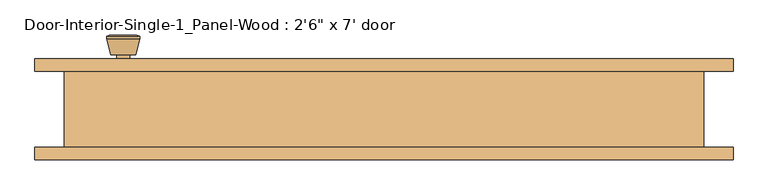
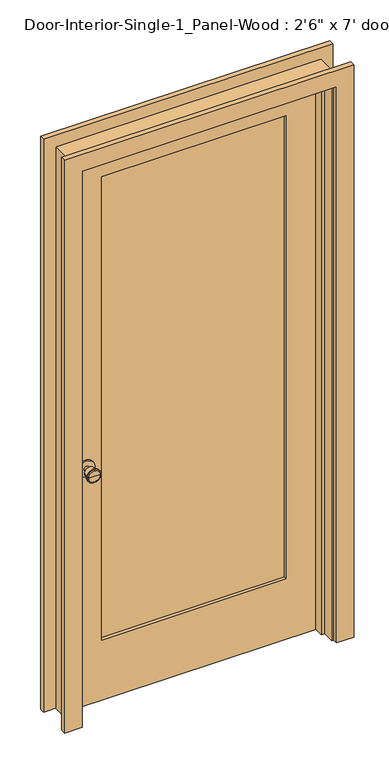
"""IFC4 building model written with IfcOpenShell, lengths in millimetres: door geometry."""

from ifc_helpers import new_model, si_unit, point, frame, frame_2d, origin, place, context, project, spatial, polyline, circle_curve, trimmed, segment, composite_curve, outline, extrude, faceted_brep, source, transform, mapped, element, save
from ifc_brep_helpers import plane_surface, cylinder_surface, revolved_surface, advanced_brep


def door_3c6ab76a(model_context):
    return source(origin(), model_context, "Body", "SolidModel", [
        advanced_brep(
        [(-393.7, 13.05, 914.4), (-383.7, 13.05, 914.4), (-403.7, 13.05, 914.4), (-373.2241324, -35.95, 914.4), (-393.7, -35.95, 914.4), (-414.1758676, -35.95, 914.4), (-368.7, -34.1221319, 914.4), (-418.7, -34.1221319, 914.4), (-368.7, -30.6584537, 914.4), (-418.7, -30.6584537, 914.4), (-375.063764, -5.95, 914.4), (-412.336236, -5.95, 914.4), (-383.7, -5.95, 914.4), (-403.7, -5.95, 914.4)],
        [
            (0, 1),
            (1, 2, circle_curve(frame((-393.7, 13.05, 914.4), z_axis=(0.0, 1.0, 0.0), x_axis=(-1.0, 0.0, 0.0)), 10.0)),
            (2, 0),
            (2, 1, circle_curve(frame((-393.7, 13.05, 914.4), z_axis=(0.0, 1.0, 0.0), x_axis=(-1.0, 0.0, 0.0)), 10.0)),
            (3, 4),
            (4, 5),
            (5, 3, circle_curve(frame((-393.7, -35.95, 914.4), z_axis=(0.0, -1.0, 0.0), x_axis=(-1.0, 0.0, 0.0)), 20.4758676)),
            (3, 5, circle_curve(frame((-393.7, -35.95, 914.4), z_axis=(0.0, -1.0, 0.0), x_axis=(-1.0, 0.0, 0.0)), 20.4758676)),
            (6, 3),
            (5, 7),
            (7, 6, circle_curve(frame((-393.7, -34.1221319, 914.4), z_axis=(0.0, -1.0, 0.0), x_axis=(-1.0, 0.0, 0.0)), 25.0)),
            (6, 7, circle_curve(frame((-393.7, -34.1221319, 914.4), z_axis=(0.0, -1.0, 0.0), x_axis=(-1.0, 0.0, 0.0)), 25.0)),
            (8, 6),
            (7, 9),
            (9, 8, circle_curve(frame((-393.7, -30.6584537, 914.4), z_axis=(0.0, -1.0, 0.0), x_axis=(-1.0, 0.0, 0.0)), 25.0)),
            (8, 9, circle_curve(frame((-393.7, -30.6584537, 914.4), z_axis=(0.0, -1.0, 0.0), x_axis=(-1.0, 0.0, 0.0)), 25.0)),
            (10, 8),
            (9, 11),
            (11, 10, circle_curve(frame((-393.7, -5.95, 914.4), z_axis=(0.0, -1.0, 0.0), x_axis=(-1.0, 0.0, 0.0)), 18.636236)),
            (10, 11, circle_curve(frame((-393.7, -5.95, 914.4), z_axis=(0.0, -1.0, 0.0), x_axis=(-1.0, 0.0, 0.0)), 18.636236)),
            (12, 10),
            (11, 13),
            (13, 12, circle_curve(frame((-393.7, -5.95, 914.4), z_axis=(0.0, -1.0, 0.0), x_axis=(-1.0, 0.0, 0.0)), 10.0)),
            (12, 13, circle_curve(frame((-393.7, -5.95, 914.4), z_axis=(0.0, -1.0, 0.0), x_axis=(-1.0, 0.0, 0.0)), 10.0)),
            (1, 12),
            (13, 2),
        ],
        [
            plane_surface(frame((-393.7, 13.05, 914.4), z_axis=(0.0, 1.0, 0.0), x_axis=(-1.0, 0.0, 0.0))),
            plane_surface(frame((-393.7, -35.95, 914.4), z_axis=(0.0, -1.0, 0.0), x_axis=(-1.0, 0.0, 0.0))),
            revolved_surface(polyline([(-414.1758676, -35.95, 914.4), (-418.7, -34.1221319, 914.4)]), (-393.7, 13.05, 914.4), (0.0, 1.0, 0.0)),
            cylinder_surface(frame((-393.7, 13.05, 914.4), z_axis=(0.0, 1.0, 0.0), x_axis=(-1.0, 0.0, 0.0)), 25.0),
            revolved_surface(polyline([(-418.7, -30.6584537, 914.4), (-412.336236, -5.95, 914.4)]), (-393.7, 13.05, 914.4), (0.0, 1.0, 0.0)),
            plane_surface(frame((-393.7, -5.95, 914.4), z_axis=(0.0, 1.0, 0.0), x_axis=(-1.0, 0.0, 0.0))),
            cylinder_surface(frame((-393.7, 13.05, 914.4), z_axis=(0.0, 1.0, 0.0), x_axis=(-1.0, 0.0, 0.0)), 10.0),
        ],
        [
            (0, [[1, 2, 3]]),
            (0, [[-3, 4, -1]]),
            (1, [[5, 6, 7]]),
            (1, [[-6, -5, 8]]),
            (2, [[9, -7, 10, 11]]),
            (2, [[-10, -8, -9, 12]]),
            (3, [[13, -11, 14, 15]]),
            (3, [[-14, -12, -13, 16]]),
            (4, [[17, -15, 18, 19]]),
            (4, [[-18, -16, -17, 20]]),
            (5, [[21, -19, 22, 23]]),
            (5, [[-22, -20, -21, 24]]),
            (6, [[25, -23, 26, -2]]),
            (6, [[-26, -24, -25, -4]]),
        ],
    ),
        extrude(outline(composite_curve([segment(trimmed(circle_curve(frame_2d((914.4, -393.7)), 30.0), [point((914.4, -423.7))], [point((914.4, -363.7))], False, "CARTESIAN"), True, "CONTINUOUS"), segment(trimmed(circle_curve(frame_2d((914.4, -393.7)), 30.0), [point((914.4, -363.7))], [point((914.4, -423.7))], False, "CARTESIAN"), True, "CONTINUOUS")], self_intersect=False)), frame((0.0, 13.05, 0.0), z_axis=(0.0, 1.0, 0.0), x_axis=(0.0, 0.0, 1.0)), (0.0, 0.0, 1.0), 6.0),
        advanced_brep(
        [(-393.7, 59.975, 914.4), (-403.7, 59.975, 914.4), (-383.7, 59.975, 914.4), (-373.2241324, 108.975, 914.4), (-414.1758676, 108.975, 914.4), (-393.7, 108.975, 914.4), (-368.7, 107.1471319, 914.4), (-418.7, 107.1471319, 914.4), (-368.7, 103.6834537, 914.4), (-418.7, 103.6834537, 914.4), (-375.063764, 78.975, 914.4), (-412.336236, 78.975, 914.4), (-383.7, 78.975, 914.4), (-403.7, 78.975, 914.4)],
        [
            (0, 1),
            (1, 2, circle_curve(frame((-393.7, 59.975, 914.4), z_axis=(0.0, -1.0, 0.0), x_axis=(-1.0, 0.0, 0.0)), 10.0)),
            (2, 0),
            (2, 1, circle_curve(frame((-393.7, 59.975, 914.4), z_axis=(0.0, -1.0, 0.0), x_axis=(-1.0, 0.0, 0.0)), 10.0)),
            (3, 4, circle_curve(frame((-393.7, 108.975, 914.4), z_axis=(0.0, 1.0, 0.0), x_axis=(-1.0, 0.0, 0.0)), 20.4758676)),
            (4, 5),
            (5, 3),
            (4, 3, circle_curve(frame((-393.7, 108.975, 914.4), z_axis=(0.0, 1.0, 0.0), x_axis=(-1.0, 0.0, 0.0)), 20.4758676)),
            (6, 7, circle_curve(frame((-393.7, 107.1471319, 914.4), z_axis=(0.0, 1.0, 0.0), x_axis=(-1.0, 0.0, 0.0)), 25.0)),
            (7, 4),
            (3, 6),
            (7, 6, circle_curve(frame((-393.7, 107.1471319, 914.4), z_axis=(0.0, 1.0, 0.0), x_axis=(-1.0, 0.0, 0.0)), 25.0)),
            (8, 9, circle_curve(frame((-393.7, 103.6834537, 914.4), z_axis=(0.0, 1.0, 0.0), x_axis=(-1.0, 0.0, 0.0)), 25.0)),
            (9, 7),
            (6, 8),
            (9, 8, circle_curve(frame((-393.7, 103.6834537, 914.4), z_axis=(0.0, 1.0, 0.0), x_axis=(-1.0, 0.0, 0.0)), 25.0)),
            (10, 11, circle_curve(frame((-393.7, 78.975, 914.4), z_axis=(0.0, 1.0, 0.0), x_axis=(-1.0, 0.0, 0.0)), 18.636236)),
            (11, 9),
            (8, 10),
            (11, 10, circle_curve(frame((-393.7, 78.975, 914.4), z_axis=(0.0, 1.0, 0.0), x_axis=(-1.0, 0.0, 0.0)), 18.636236)),
            (12, 13, circle_curve(frame((-393.7, 78.975, 914.4), z_axis=(0.0, 1.0, 0.0), x_axis=(-1.0, 0.0, 0.0)), 10.0)),
            (13, 11),
            (10, 12),
            (13, 12, circle_curve(frame((-393.7, 78.975, 914.4), z_axis=(0.0, 1.0, 0.0), x_axis=(-1.0, 0.0, 0.0)), 10.0)),
            (1, 13),
            (12, 2),
        ],
        [
            plane_surface(frame((-393.7, 59.975, 914.4), z_axis=(0.0, -1.0, 0.0), x_axis=(-1.0, 0.0, 0.0))),
            plane_surface(frame((-393.7, 108.975, 914.4), z_axis=(0.0, 1.0, 0.0), x_axis=(-1.0, 0.0, 0.0))),
            revolved_surface(polyline([(-414.1758676, 108.975, 914.4), (-418.7, 107.1471319, 914.4)]), (-393.7, 59.975, 914.4), (0.0, -1.0, 0.0)),
            cylinder_surface(frame((-393.7, 59.975, 914.4), z_axis=(0.0, -1.0, 0.0), x_axis=(-1.0, 0.0, 0.0)), 25.0),
            revolved_surface(polyline([(-418.7, 103.6834537, 914.4), (-412.336236, 78.975, 914.4)]), (-393.7, 59.975, 914.4), (0.0, -1.0, 0.0)),
            plane_surface(frame((-393.7, 78.975, 914.4), z_axis=(0.0, -1.0, 0.0), x_axis=(-1.0, 0.0, 0.0))),
            cylinder_surface(frame((-393.7, 59.975, 914.4), z_axis=(0.0, -1.0, 0.0), x_axis=(-1.0, 0.0, 0.0)), 10.0),
        ],
        [
            (0, [[1, 2, 3]]),
            (0, [[-3, 4, -1]]),
            (1, [[5, 6, 7]]),
            (1, [[8, -7, -6]]),
            (2, [[9, 10, -5, 11]]),
            (2, [[12, -11, -8, -10]]),
            (3, [[13, 14, -9, 15]]),
            (3, [[16, -15, -12, -14]]),
            (4, [[17, 18, -13, 19]]),
            (4, [[20, -19, -16, -18]]),
            (5, [[21, 22, -17, 23]]),
            (5, [[24, -23, -20, -22]]),
            (6, [[-2, 25, -21, 26]]),
            (6, [[-4, -26, -24, -25]]),
        ],
    ),
        extrude(outline(composite_curve([segment(trimmed(circle_curve(frame_2d((914.4, -393.7)), 30.0), [point((914.4, -423.7))], [point((914.4, -363.7))], False, "CARTESIAN"), True, "CONTINUOUS"), segment(trimmed(circle_curve(frame_2d((914.4, -393.7)), 30.0), [point((914.4, -363.7))], [point((914.4, -423.7))], False, "CARTESIAN"), True, "CONTINUOUS")], self_intersect=False)), frame((0.0, 53.975, 0.0), z_axis=(0.0, 1.0, 0.0), x_axis=(0.0, 0.0, 1.0)), (0.0, 0.0, 1.0), 6.0),
        faceted_brep([(482.6, 53.975, 0.0), (482.6, -60.325, 0.0), (457.2, -60.325, 0.0), (457.2, -15.875, 0.0), (444.5, -15.875, 0.0), (444.5, 19.05, 0.0), (457.2, 19.05, 0.0), (457.2, 53.975, 0.0), (482.6, 53.975, 2159.0), (482.6, -60.325, 2159.0), (-482.6, -60.325, 2159.0), (-482.6, -60.325, 0.0), (-457.2, -60.325, 0.0), (-457.2, -60.325, 2133.6), (457.2, -60.325, 2133.6), (457.2, -15.875, 2133.6), (-457.2, -15.875, 2133.6), (-457.2, -15.875, 0.0), (-444.5, -15.875, 0.0), (-444.5, -15.875, 2120.9), (444.5, -15.875, 2120.9), (444.5, 19.05, 2120.9), (-444.5, 19.05, 2120.9), (-444.5, 19.05, 0.0), (-457.2, 19.05, 0.0), (-457.2, 19.05, 2133.6), (457.2, 19.05, 2133.6), (457.2, 53.975, 2133.6), (-457.2, 53.975, 2133.6), (-457.2, 53.975, 0.0), (-482.6, 53.975, 0.0), (-482.6, 53.975, 2159.0)], [[[0, 1, 2, 3, 4, 5, 6, 7]], [[1, 0, 8, 9]], [[2, 1, 9, 10, 11, 12, 13, 14]], [[3, 2, 14, 15]], [[4, 3, 15, 16, 17, 18, 19, 20]], [[5, 4, 20, 21]], [[6, 5, 21, 22, 23, 24, 25, 26]], [[7, 6, 26, 27]], [[0, 7, 27, 28, 29, 30, 31, 8]], [[9, 8, 31, 10]], [[15, 14, 13, 16]], [[21, 20, 19, 22]], [[27, 26, 25, 28]], [[30, 29, 24, 23, 18, 17, 12, 11]], [[10, 31, 30, 11]], [[16, 13, 12, 17]], [[22, 19, 18, 23]], [[28, 25, 24, 29]]]),
        extrude(outline(polyline([(2133.6, -457.2), (0.0, -457.2), (0.0, 457.2), (2133.6, 457.2), (2133.6, -457.2)]), holes=[polyline([(2014.5375, -336.55), (2014.5375, 336.55), (231.775, 336.55), (231.775, -336.55), (2014.5375, -336.55)])]), frame((0.0, 19.05, 0.0), z_axis=(0.0, 1.0, 0.0), x_axis=(0.0, 0.0, 1.0)), (0.0, 0.0, 1.0), 34.925),
        extrude(outline(polyline([(336.55, 30.6916667), (-336.55, 30.6916667), (-336.55, 42.3333333), (336.55, 42.3333333), (336.55, 30.6916667)])), frame((0.0, 0.0, 231.775), z_axis=(0.0, 0.0, 1.0), x_axis=(1.0, 0.0, 0.0)), (0.0, 0.0, 1.0), 1782.7625),
        extrude(outline(polyline([(0.0, 463.55), (0.0, 527.05), (2203.45, 527.05), (2203.45, -527.05), (0.0, -527.05), (0.0, -463.55), (2139.95, -463.55), (2139.95, 463.55), (0.0, 463.55)])), frame((0.0, 53.975, 0.0), z_axis=(0.0, 1.0, 0.0), x_axis=(0.0, 0.0, 1.0)), (0.0, 0.0, 1.0), 19.05),
        extrude(outline(polyline([(0.0, 463.55), (0.0, 527.05), (2203.45, 527.05), (2203.45, -527.05), (0.0, -527.05), (0.0, -463.55), (2139.95, -463.55), (2139.95, 463.55), (0.0, 463.55)])), frame((0.0, -79.375, 0.0), z_axis=(0.0, 1.0, 0.0), x_axis=(0.0, 0.0, 1.0)), (0.0, 0.0, 1.0), 19.05),
    ])


if __name__ == "__main__":
    model = new_model("IFC4")
    model_context = context("Model", 3, world=origin())
    ifc_project = project(units=[si_unit("LENGTHUNIT", "METRE", prefix="MILLI")], contexts=[model_context])
    site = spatial("IfcSite", under=ifc_project)
    building = spatial("IfcBuilding", under=site)
    placement = place(None, origin())
    door_shape = door_3c6ab76a(model_context)
    element("IfcDoor", 1, ObjectType="Door-Interior-Single-1_Panel-Wood : 2'6\" x 7' door", at=placement, inside=building, context=model_context, shape_type="MappedRepresentation", body=[
        mapped(door_shape, transform((0.0, 0.0, 0.0), x_axis=(1.0, 0.0, 0.0), y_axis=(0.0, 1.0, 0.0), z_axis=(0.0, 0.0, 1.0))),
    ])
    save(model, "model.ifc")

# Revit data of these elements
# Type "Door-Interior-Single-1_Panel-Wood : 2'6\" x 7' door"
#   Type Mark = "9"
#   Assembly Code = "C1020300"
#   Analytic Construction = "Wooden"
#   Top Rail = 0' - 4 11/16"
#   Thickness = 0' - 1 3/8"
#   Thermal Resistance (R) = 2.5876 (h·ft²·°F)/BTU
#   Swing Angle [instance default] = 90.00°
#   Stiles = 0' - 4 3/4"
#   Rough Width = 3' - 2"
#   Rough Height = 7' - 1"
#   Height = 7' - 0"
#   Width = 3' - 0"
#   Heat Transfer Coefficient (U) = 0.3865 BTU/(h·ft²·°F)
#   Bottom Rail = 0' - 9 1/8"
#   Trim Material = Cherry
#   Panel Material = Cherry
#   Frame Material = Cherry
#   Door Handle Material = Aluminum
#   Visual Light Transmittance = 0
#   Solar Heat Gain Coefficient = 0
#   Wall Closure = (empty or 0)
#   Function = (empty or 0)
# Element 1 (IfcDoor, "Door-Interior-Single-1_Panel-Wood : 2'6\" x 7' door")
#   Materials on its faces: "Cherry", "Aluminum"
# Materials
#   "Cherry": class "Wood", colour RGB 226 177 128, transparency 0, Description = "Prunus Serotina", Cost = 0
#   "Aluminum": class "Metal", colour RGB 247 247 247, transparency 0, Description = "Aluminum 6061", Cost = 0
